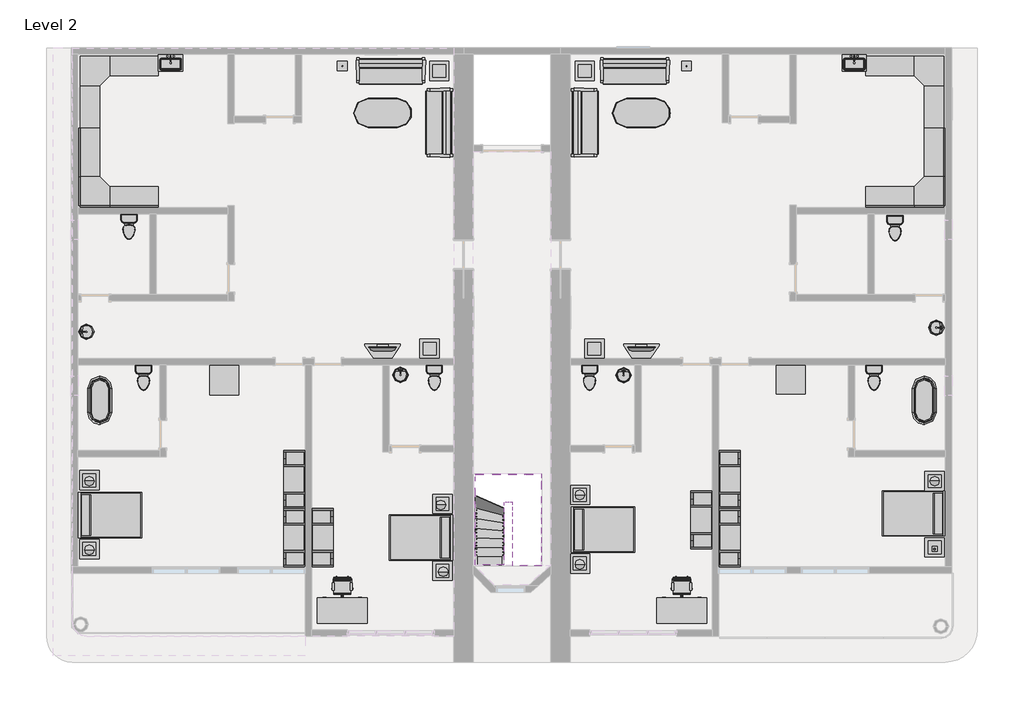
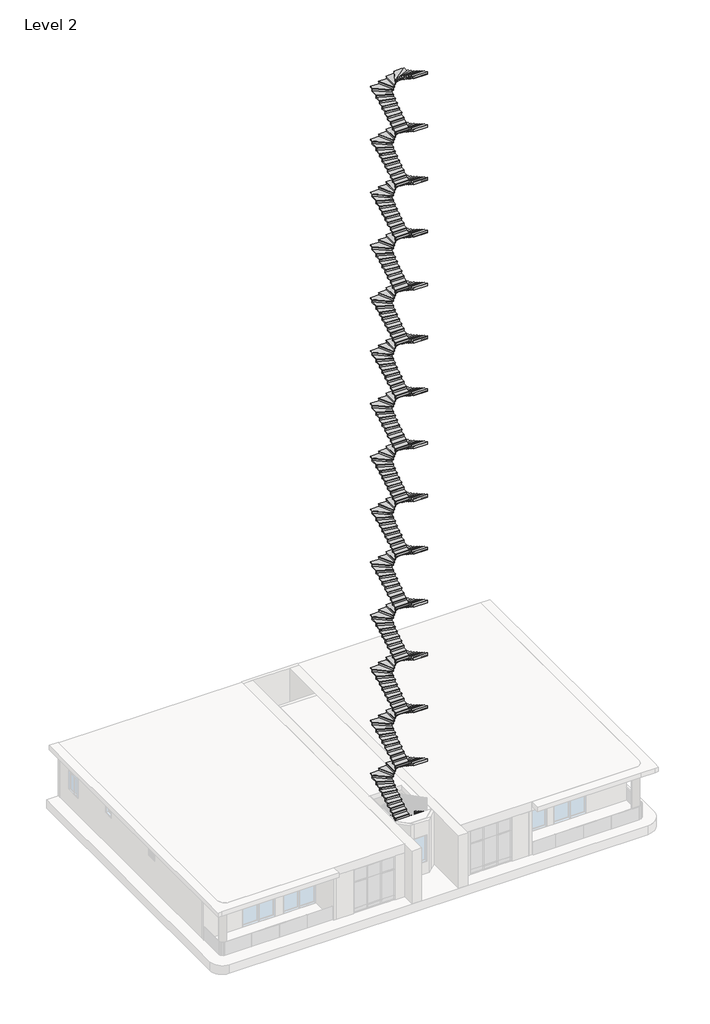
# One storey, part 5 of 5: 42 furniture elements, 16 stair flights, 14 flow terminals, 10 light fixtures.
"""IFC4 building model written with IfcOpenShell, lengths in millimetres."""

from ifc_helpers import new_model, si_unit, origin, place, context, project, spatial, transform, mapped, element, save
from components import flow_terminal_38af2918, flow_terminal_d49f872f, toilet_domestic_3d_toilet_domestic_3d_f7549cf7, toilet_domestic_3d_toilet_domestic_3d_183bbd19, flow_terminal_b374fae2, furniture_07436f11, furniture_096e7f55, chair_task_arms_chair_task_arms_fa5a08ef, furniture_072f6425, furniture_cf0b6580, furniture_aff9b2fb, furniture_56245f3a, tv_stand_tv_stand_6ce107e5, furniture_b5c51a22, furniture_2c34a4f9, furniture_4d44e21c, furniture_45e3acac, light_fixture_100w_120v_8564026f, table_lamp_hemispheric_60w_120v_02721d88, stair_flight_836873dd, stair_flight_696a7c4e, stair_flight_777e5497, stair_flight_57db1963, stair_flight_2efad17c, stair_flight_652fc51c, stair_flight_77a7b7b7, stair_flight_6c5b5e9d, stair_flight_464fb83d, stair_flight_aac49ba0, stair_flight_d4b8cc4c, stair_flight_2169dd6b, stair_flight_c7d98fdd, stair_flight_11ab74ad, stair_flight_b3d82c80

model = new_model("IFC4")

# Units and contexts
model_context = context("Model", 3, world=origin())
ifc_project = project(units=[si_unit("LENGTHUNIT", "METRE", prefix="MILLI")], contexts=[model_context])

# Site, building, storey
site = spatial("IfcSite", under=ifc_project)
building = spatial("IfcBuilding", under=site)
storey = spatial("IfcBuildingStorey", under=building, Name="Level 2", Elevation=3657.6)

# Flow terminals
placement = place(None, origin())
flow_terminal_shape = flow_terminal_38af2918(model_context)
element("IfcFlowTerminal", 1, ObjectType="Sink Kitchen-Single : 30\" x 21\"", at=placement, inside=storey, context=model_context, shape_type="MappedRepresentation", body=[
    mapped(flow_terminal_shape, transform((-15540.388011, 11239.7304546, 3657.6), x_axis=(1.0, 0.0, 0.0), y_axis=(0.0, 1.0, 0.0), z_axis=(0.0, 0.0, 1.0))),
])
element("IfcFlowTerminal", 2, ObjectType="Sink Kitchen-Single : 30\" x 21\"", at=placement, inside=storey, context=model_context, shape_type="MappedRepresentation", body=[
    mapped(flow_terminal_shape, transform((5948.011989, 11239.7304546, 3657.6), x_axis=(1.0, 0.0, 0.0), y_axis=(0.0, 1.0, 0.0), z_axis=(0.0, 0.0, 1.0))),
])
flow_terminal_2_shape = flow_terminal_d49f872f(model_context)
element("IfcFlowTerminal", 3, ObjectType="Sink Vanity-Round : 19\" x 19\"", at=placement, inside=storey, context=model_context, shape_type="MappedRepresentation", body=[
    mapped(flow_terminal_2_shape, transform((-18084.6070794, 2687.2241152, 3657.6), x_axis=(0.0, 1.0000000000000002, 0.0), y_axis=(-1.0000000000000002, 0.0, 0.0), z_axis=(0.0, 0.0, 1.0))),
])
element("IfcFlowTerminal", 4, ObjectType="Sink Vanity-Round : 19\" x 19\"", at=placement, inside=storey, context=model_context, shape_type="MappedRepresentation", body=[
    mapped(flow_terminal_2_shape, transform((8462.2249463, 3007.5275963, 3657.6), x_axis=(0.0, -1.0000000000000004, 0.0), y_axis=(1.0000000000000004, 0.0, 0.0), z_axis=(0.0, 0.0, 1.0))),
])
element("IfcFlowTerminal", 5, ObjectType="Sink Vanity-Round : 19\" x 19\"", at=placement, inside=storey, context=model_context, shape_type="MappedRepresentation", body=[
    mapped(flow_terminal_2_shape, transform((-8395.050511, 1341.8921141, 3657.6), x_axis=(1.0, 0.0, 0.0), y_axis=(0.0, 1.0, 0.0), z_axis=(0.0, 0.0, 1.0))),
])
element("IfcFlowTerminal", 6, ObjectType="Sink Vanity-Round : 19\" x 19\"", at=placement, inside=storey, context=model_context, shape_type="MappedRepresentation", body=[
    mapped(flow_terminal_2_shape, transform((-1384.650511, 1331.0855344, 3657.6), x_axis=(1.0, 0.0, 0.0), y_axis=(0.0, 1.0, 0.0), z_axis=(0.0, 0.0, 1.0))),
])
toilet_domestic_3d_toilet_domestic_3d_shape = toilet_domestic_3d_toilet_domestic_3d_f7549cf7(model_context)
toilet_domestic_3d_toilet_domestic_3d_2_shape = toilet_domestic_3d_toilet_domestic_3d_183bbd19(model_context)
element("IfcFlowTerminal", 7, ObjectType="Toilet-Domestic-3D : Toilet-Domestic-3D", at=placement, inside=storey, context=model_context, shape_type="MappedRepresentation", body=[
    mapped(toilet_domestic_3d_toilet_domestic_3d_shape, transform((6586.0012296, 1247.7798284, 3657.6), x_axis=(1.0, 0.0, 0.0), y_axis=(0.0, 1.0, 0.0), z_axis=(0.0, 0.0, 1.0))),
    mapped(toilet_domestic_3d_toilet_domestic_3d_2_shape, transform((6586.0012296, 1247.7798284, 3657.6), x_axis=(1.0, 0.0, 0.0), y_axis=(0.0, 1.0, 0.0), z_axis=(0.0, 0.0, 1.0))),
])
element("IfcFlowTerminal", 8, ObjectType="Toilet-Domestic-3D : Toilet-Domestic-3D", at=placement, inside=storey, context=model_context, shape_type="MappedRepresentation", body=[
    mapped(toilet_domestic_3d_toilet_domestic_3d_shape, transform((-2354.7987704, 1247.7798284, 3657.6), x_axis=(1.0, 0.0, 0.0), y_axis=(0.0, 1.0, 0.0), z_axis=(0.0, 0.0, 1.0))),
    mapped(toilet_domestic_3d_toilet_domestic_3d_2_shape, transform((-2354.7987704, 1247.7798284, 3657.6), x_axis=(1.0, 0.0, 0.0), y_axis=(0.0, 1.0, 0.0), z_axis=(0.0, 0.0, 1.0))),
])
element("IfcFlowTerminal", 9, ObjectType="Toilet-Domestic-3D : Toilet-Domestic-3D", at=placement, inside=storey, context=model_context, shape_type="MappedRepresentation", body=[
    mapped(toilet_domestic_3d_toilet_domestic_3d_shape, transform((-16375.5987704, 1247.7798284, 3657.6), x_axis=(1.0, 0.0, 0.0), y_axis=(0.0, 1.0, 0.0), z_axis=(0.0, 0.0, 1.0))),
    mapped(toilet_domestic_3d_toilet_domestic_3d_2_shape, transform((-16375.5987704, 1247.7798284, 3657.6), x_axis=(1.0, 0.0, 0.0), y_axis=(0.0, 1.0, 0.0), z_axis=(0.0, 0.0, 1.0))),
])
element("IfcFlowTerminal", 10, ObjectType="Toilet-Domestic-3D : Toilet-Domestic-3D", at=placement, inside=storey, context=model_context, shape_type="MappedRepresentation", body=[
    mapped(toilet_domestic_3d_toilet_domestic_3d_shape, transform((-16832.7987704, 5997.5798284, 3657.6), x_axis=(1.0, 0.0, 0.0), y_axis=(0.0, 1.0, 0.0), z_axis=(0.0, 0.0, 1.0))),
    mapped(toilet_domestic_3d_toilet_domestic_3d_2_shape, transform((-16832.7987704, 5997.5798284, 3657.6), x_axis=(1.0, 0.0, 0.0), y_axis=(0.0, 1.0, 0.0), z_axis=(0.0, 0.0, 1.0))),
])
element("IfcFlowTerminal", 11, ObjectType="Toilet-Domestic-3D : Toilet-Domestic-3D", at=placement, inside=storey, context=model_context, shape_type="MappedRepresentation", body=[
    mapped(toilet_domestic_3d_toilet_domestic_3d_shape, transform((7246.4012296, 5946.7798284, 3657.6), x_axis=(1.0, 0.0, 0.0), y_axis=(0.0, 1.0, 0.0), z_axis=(0.0, 0.0, 1.0))),
    mapped(toilet_domestic_3d_toilet_domestic_3d_2_shape, transform((7246.4012296, 5946.7798284, 3657.6), x_axis=(1.0, 0.0, 0.0), y_axis=(0.0, 1.0, 0.0), z_axis=(0.0, 0.0, 1.0))),
])
element("IfcFlowTerminal", 12, ObjectType="Toilet-Domestic-3D : Toilet-Domestic-3D", at=placement, inside=storey, context=model_context, shape_type="MappedRepresentation", body=[
    mapped(toilet_domestic_3d_toilet_domestic_3d_shape, transform((-7231.5987704, 1247.7798284, 3657.6), x_axis=(1.0, 0.0, 0.0), y_axis=(0.0, 1.0, 0.0), z_axis=(0.0, 0.0, 1.0))),
    mapped(toilet_domestic_3d_toilet_domestic_3d_2_shape, transform((-7231.5987704, 1247.7798284, 3657.6), x_axis=(1.0, 0.0, 0.0), y_axis=(0.0, 1.0, 0.0), z_axis=(0.0, 0.0, 1.0))),
])
flow_terminal_3_shape = flow_terminal_b374fae2(model_context)
element("IfcFlowTerminal", 13, ObjectType="Tub-Free Standing-3D : 30\" x 60\"", at=placement, inside=storey, context=model_context, shape_type="MappedRepresentation", body=[
    mapped(flow_terminal_3_shape, transform((-17747.1987704, 624.8758558, 3657.6), x_axis=(1.0, 0.0, 0.0), y_axis=(0.0, 1.0, 0.0), z_axis=(0.0, 0.0, 1.0))),
])
element("IfcFlowTerminal", 14, ObjectType="Tub-Free Standing-3D : 30\" x 60\"", at=placement, inside=storey, context=model_context, shape_type="MappedRepresentation", body=[
    mapped(flow_terminal_3_shape, transform((8160.8012296, 624.8758558, 3657.6), x_axis=(1.0, 0.0, 0.0), y_axis=(0.0, 1.0, 0.0), z_axis=(0.0, 0.0, 1.0))),
])

# Furniture
furniture_shape = furniture_07436f11(model_context)
element("IfcFurniture", 15, ObjectType="96\" x 96\"", at=placement, inside=storey, context=model_context, shape_type="MappedRepresentation", body=[
    mapped(furniture_shape, transform((-18275.8670182, 11991.0988634, 3657.6), x_axis=(1.0, 0.0, 0.0), y_axis=(0.0, 1.0, 0.0), z_axis=(0.0, 0.0, 1.0))),
])
element("IfcFurniture", 16, ObjectType="96\" x 96\"", at=placement, inside=storey, context=model_context, shape_type="MappedRepresentation", body=[
    mapped(furniture_shape, transform((9316.2242372, 11364.3441035, 3657.6), x_axis=(0.0, -1.0000000000000004, 0.0), y_axis=(1.0000000000000004, 0.0, 0.0), z_axis=(0.0, 0.0, 1.0))),
])
furniture_2_shape = furniture_096e7f55(model_context)
element("IfcFurniture", 17, ObjectType="Bed-Shaker : Double 56\" x 78\"", at=placement, inside=storey, context=model_context, shape_type="MappedRepresentation", body=[
    mapped(furniture_2_shape, transform((-18407.5987704, -2962.8741442, 3657.6), x_axis=(0.0, 1.0, 0.0), y_axis=(-1.0, 0.0, 0.0), z_axis=(0.0, 0.0, 1.0))),
])
element("IfcFurniture", 18, ObjectType="Bed-Shaker : Double 56\" x 78\"", at=placement, inside=storey, context=model_context, shape_type="MappedRepresentation", body=[
    mapped(furniture_2_shape, transform((-6672.7987704, -3712.1741442, 3657.6), x_axis=(0.0, -1.0, 0.0), y_axis=(1.0, 0.0, 0.0), z_axis=(0.0, 0.0, 1.0))),
])
element("IfcFurniture", 19, ObjectType="Bed-Shaker : Double 56\" x 78\"", at=placement, inside=storey, context=model_context, shape_type="MappedRepresentation", body=[
    mapped(furniture_2_shape, transform((-2913.5987704, -3420.0741442, 3657.6), x_axis=(0.0, 1.0000000000000002, 0.0), y_axis=(-1.0000000000000002, 0.0, 0.0), z_axis=(0.0, 0.0, 1.0))),
])
element("IfcFurniture", 20, ObjectType="Bed-Shaker : Double 56\" x 78\"", at=placement, inside=storey, context=model_context, shape_type="MappedRepresentation", body=[
    mapped(furniture_2_shape, transform((8821.2012296, -2950.1741442, 3657.6), x_axis=(0.0, -1.0, 0.0), y_axis=(1.0, 0.0, 0.0), z_axis=(0.0, 0.0, 1.0))),
])
chair_task_arms_chair_task_arms_shape = chair_task_arms_chair_task_arms_fa5a08ef(model_context)
element("IfcFurniture", 21, ObjectType="Chair-Task Arms : Chair-Task Arms", at=placement, inside=storey, context=model_context, shape_type="MappedRepresentation", body=[
    mapped(chair_task_arms_chair_task_arms_shape, transform((681.7920493, -5184.3566833, 3657.6), x_axis=(-1.0000000000000002, 0.0, 0.0), y_axis=(0.0, -1.0000000000000002, 0.0), z_axis=(0.0, 0.0, 1.0))),
])
element("IfcFurniture", 22, ObjectType="Chair-Task Arms : Chair-Task Arms", at=placement, inside=storey, context=model_context, shape_type="MappedRepresentation", body=[
    mapped(chair_task_arms_chair_task_arms_shape, transform((-9986.2079507, -5184.3566833, 3657.6), x_axis=(-1.0, 0.0, 0.0), y_axis=(0.0, -1.0, 0.0), z_axis=(0.0, 0.0, 1.0))),
])
furniture_3_shape = furniture_072f6425(model_context)
element("IfcFurniture", 23, ObjectType="Desk : 60\" x 30\"", at=placement, inside=storey, context=model_context, shape_type="MappedRepresentation", body=[
    mapped(furniture_3_shape, transform((-10889.1987704, -6371.702585, 3657.6), x_axis=(1.0, 0.0, 0.0), y_axis=(0.0, 1.0, 0.0), z_axis=(0.0, 0.0, 1.0))),
])
element("IfcFurniture", 24, ObjectType="Desk : 60\" x 30\"", at=placement, inside=storey, context=model_context, shape_type="MappedRepresentation", body=[
    mapped(furniture_3_shape, transform((-221.1987704, -6371.702585, 3657.6), x_axis=(1.0, 0.0, 0.0), y_axis=(0.0, 1.0, 0.0), z_axis=(0.0, 0.0, 1.0))),
])
furniture_4_shape = furniture_cf0b6580(model_context)
element("IfcFurniture", 25, ObjectType="Entertainment Center : 72\" x 72\" x 24\"", at=placement, inside=storey, context=model_context, shape_type="MappedRepresentation", body=[
    mapped(furniture_4_shape, transform((1607.6012296, -3134.3241442, 3657.6), x_axis=(0.0, -1.0000000000000002, 0.0), y_axis=(1.0000000000000002, 0.0, 0.0), z_axis=(0.0, 0.0, 1.0))),
])
element("IfcFurniture", 26, ObjectType="Entertainment Center : 72\" x 72\" x 24\"", at=placement, inside=storey, context=model_context, shape_type="MappedRepresentation", body=[
    mapped(furniture_4_shape, transform((1607.6012296, -3693.1241442, 3657.6), x_axis=(0.0, 1.0000000000000004, 0.0), y_axis=(-1.0000000000000004, 0.0, 0.0), z_axis=(0.0, 0.0, 1.0))),
])
element("IfcFurniture", 27, ObjectType="Entertainment Center : 72\" x 72\" x 24\"", at=placement, inside=storey, context=model_context, shape_type="MappedRepresentation", body=[
    mapped(furniture_4_shape, transform((1607.6012296, -1864.3241442, 3657.6), x_axis=(0.0, 1.0000000000000004, 0.0), y_axis=(-1.0000000000000004, 0.0, 0.0), z_axis=(0.0, 0.0, 1.0))),
])
element("IfcFurniture", 28, ObjectType="Entertainment Center : 72\" x 72\" x 24\"", at=placement, inside=storey, context=model_context, shape_type="MappedRepresentation", body=[
    mapped(furniture_4_shape, transform((-11193.9987704, -3693.1241442, 3657.6), x_axis=(0.0, -1.0000000000000016, 0.0), y_axis=(1.0000000000000016, 0.0, 0.0), z_axis=(0.0, 0.0, 1.0))),
])
element("IfcFurniture", 29, ObjectType="Entertainment Center : 72\" x 72\" x 24\"", at=placement, inside=storey, context=model_context, shape_type="MappedRepresentation", body=[
    mapped(furniture_4_shape, transform((-11193.9987704, -1864.3241442, 3657.6), x_axis=(0.0, -1.0000000000000004, 0.0), y_axis=(1.0000000000000004, 0.0, 0.0), z_axis=(0.0, 0.0, 1.0))),
])
element("IfcFurniture", 30, ObjectType="Entertainment Center : 72\" x 72\" x 24\"", at=placement, inside=storey, context=model_context, shape_type="MappedRepresentation", body=[
    mapped(furniture_4_shape, transform((-11193.9987704, -3693.1241442, 3657.6), x_axis=(0.0, 1.0, 0.0), y_axis=(-1.0, 0.0, 0.0), z_axis=(0.0, 0.0, 1.0))),
])
furniture_5_shape = furniture_aff9b2fb(model_context)
element("IfcFurniture", 31, ObjectType="Sofa-Pensi : 84\"", at=placement, inside=storey, context=model_context, shape_type="MappedRepresentation", body=[
    mapped(furniture_5_shape, transform((-8881.8050204, 10710.9660197, 3657.6), x_axis=(1.0, 0.0, 0.0), y_axis=(0.0, 1.0, 0.0), z_axis=(0.0, 0.0, 1.0))),
])
element("IfcFurniture", 32, ObjectType="Sofa-Pensi : 84\"", at=placement, inside=storey, context=model_context, shape_type="MappedRepresentation", body=[
    mapped(furniture_5_shape, transform((-7356.3086065, 9641.0821058, 3657.6), x_axis=(0.0, -1.0000000000000004, 0.0), y_axis=(1.0000000000000004, 0.0, 0.0), z_axis=(0.0, 0.0, 1.0))),
])
element("IfcFurniture", 33, ObjectType="Sofa-Pensi : 84\"", at=placement, inside=storey, context=model_context, shape_type="MappedRepresentation", body=[
    mapped(furniture_5_shape, transform((-2230.0889343, 9083.8696058, 3657.6), x_axis=(0.0, 1.0000000000000002, 0.0), y_axis=(-1.0000000000000002, 0.0, 0.0), z_axis=(0.0, 0.0, 1.0))),
])
element("IfcFurniture", 34, ObjectType="Sofa-Pensi : 84\"", at=placement, inside=storey, context=model_context, shape_type="MappedRepresentation", body=[
    mapped(furniture_5_shape, transform((-1211.0050204, 10710.9660197, 3657.6), x_axis=(1.0000000000000007, 0.0, 0.0), y_axis=(0.0, 1.0000000000000007, 0.0), z_axis=(0.0, 0.0, 1.0))),
])
furniture_6_shape = furniture_56245f3a(model_context)
element("IfcFurniture", 35, ObjectType="TV - Flat Screen : 32\"", at=placement, inside=storey, context=model_context, shape_type="MappedRepresentation", body=[
    mapped(furniture_6_shape, transform((-8861.1432846, 2232.8144794, 4572.0), x_axis=(-1.0, 0.0, 0.0), y_axis=(0.0, -1.0, 0.0), z_axis=(0.0, 0.0, 1.0))),
])
element("IfcFurniture", 36, ObjectType="TV - Flat Screen : 32\"", at=placement, inside=storey, context=model_context, shape_type="MappedRepresentation", body=[
    mapped(furniture_6_shape, transform((-733.1432846, 2232.8144794, 4572.0), x_axis=(-1.0, 0.0, 0.0), y_axis=(0.0, -1.0, 0.0), z_axis=(0.0, 0.0, 1.0))),
])
tv_stand_tv_stand_shape = tv_stand_tv_stand_6ce107e5(model_context)
element("IfcFurniture", 37, ObjectType="TV Stand : TV Stand", at=placement, inside=storey, context=model_context, shape_type="MappedRepresentation", body=[
    mapped(tv_stand_tv_stand_shape, transform((-8732.0107683, 1945.6758558, 3657.6), x_axis=(-1.0000000000000002, 0.0, 0.0), y_axis=(0.0, -1.0000000000000002, 0.0), z_axis=(0.0, 0.0, 1.0))),
])
element("IfcFurniture", 38, ObjectType="TV Stand : TV Stand", at=placement, inside=storey, context=model_context, shape_type="MappedRepresentation", body=[
    mapped(tv_stand_tv_stand_shape, transform((-604.0107683, 1945.6758558, 3657.6), x_axis=(-1.0, 0.0, 0.0), y_axis=(0.0, -1.0, 0.0), z_axis=(0.0, 0.0, 1.0))),
])
furniture_7_shape = furniture_b5c51a22(model_context)
element("IfcFurniture", 39, ObjectType="Table-Coffee : 24\" x 24\" x 24\"", at=placement, inside=storey, context=model_context, shape_type="MappedRepresentation", body=[
    mapped(furniture_7_shape, transform((-7097.4645371, 10892.864778, 3657.6), x_axis=(1.0, 0.0, 0.0), y_axis=(0.0, 1.0, 0.0), z_axis=(0.0, 0.0, 1.0))),
])
element("IfcFurniture", 40, ObjectType="Table-Coffee : 24\" x 24\" x 24\"", at=placement, inside=storey, context=model_context, shape_type="MappedRepresentation", body=[
    mapped(furniture_7_shape, transform((-2525.4645371, 10892.864778, 3657.6), x_axis=(1.0, 0.0, 0.0), y_axis=(0.0, 1.0, 0.0), z_axis=(0.0, 0.0, 1.0))),
])
element("IfcFurniture", 41, ObjectType="Table-Coffee : 24\" x 24\" x 24\"", at=placement, inside=storey, context=model_context, shape_type="MappedRepresentation", body=[
    mapped(furniture_7_shape, transform((-7402.2645371, 2155.264778, 3657.6), x_axis=(1.0, 0.0, 0.0), y_axis=(0.0, 1.0, 0.0), z_axis=(0.0, 0.0, 1.0))),
])
element("IfcFurniture", 42, ObjectType="Table-Coffee : 24\" x 24\" x 24\"", at=placement, inside=storey, context=model_context, shape_type="MappedRepresentation", body=[
    mapped(furniture_7_shape, transform((-2220.6645371, 2155.264778, 3657.6), x_axis=(1.0, 0.0, 0.0), y_axis=(0.0, 1.0, 0.0), z_axis=(0.0, 0.0, 1.0))),
])
element("IfcFurniture", 43, ObjectType="Table-Coffee : 24\" x 24\" x 24\"", at=placement, inside=storey, context=model_context, shape_type="MappedRepresentation", body=[
    mapped(furniture_7_shape, transform((-2677.8645371, -4601.135222, 3657.6), x_axis=(1.0, 0.0, 0.0), y_axis=(0.0, 1.0, 0.0), z_axis=(0.0, 0.0, 1.0))),
])
element("IfcFurniture", 44, ObjectType="Table-Coffee : 24\" x 24\" x 24\"", at=placement, inside=storey, context=model_context, shape_type="MappedRepresentation", body=[
    mapped(furniture_7_shape, transform((-18095.6645371, -4143.935222, 3657.6), x_axis=(1.0, 0.0, 0.0), y_axis=(0.0, 1.0, 0.0), z_axis=(0.0, 0.0, 1.0))),
])
element("IfcFurniture", 45, ObjectType="Table-Coffee : 24\" x 24\" x 24\"", at=placement, inside=storey, context=model_context, shape_type="MappedRepresentation", body=[
    mapped(furniture_7_shape, transform((-18095.6645371, -1984.935222, 3657.6), x_axis=(1.0, 0.0, 0.0), y_axis=(0.0, 1.0, 0.0), z_axis=(0.0, 0.0, 1.0))),
])
element("IfcFurniture", 46, ObjectType="Table-Coffee : 24\" x 24\" x 24\"", at=placement, inside=storey, context=model_context, shape_type="MappedRepresentation", body=[
    mapped(furniture_7_shape, transform((-2677.8645371, -2442.135222, 3657.6), x_axis=(1.0, 0.0, 0.0), y_axis=(0.0, 1.0, 0.0), z_axis=(0.0, 0.0, 1.0))),
])
element("IfcFurniture", 47, ObjectType="Table-Coffee : 24\" x 24\" x 24\"", at=placement, inside=storey, context=model_context, shape_type="MappedRepresentation", body=[
    mapped(furniture_7_shape, transform((8472.7354629, -4093.135222, 3657.6), x_axis=(1.0, 0.0, 0.0), y_axis=(0.0, 1.0, 0.0), z_axis=(0.0, 0.0, 1.0))),
])
element("IfcFurniture", 48, ObjectType="Table-Coffee : 24\" x 24\" x 24\"", at=placement, inside=storey, context=model_context, shape_type="MappedRepresentation", body=[
    mapped(furniture_7_shape, transform((8472.7354629, -2010.335222, 3657.6), x_axis=(1.0, 0.0, 0.0), y_axis=(0.0, 1.0, 0.0), z_axis=(0.0, 0.0, 1.0))),
])
element("IfcFurniture", 49, ObjectType="Table-Coffee : 24\" x 24\" x 24\"", at=placement, inside=storey, context=model_context, shape_type="MappedRepresentation", body=[
    mapped(furniture_7_shape, transform((-6995.8645371, -4832.0414601, 3657.6), x_axis=(1.0, 0.0, 0.0), y_axis=(0.0, 1.0, 0.0), z_axis=(0.0, 0.0, 1.0))),
])
element("IfcFurniture", 50, ObjectType="Table-Coffee : 24\" x 24\" x 24\"", at=placement, inside=storey, context=model_context, shape_type="MappedRepresentation", body=[
    mapped(furniture_7_shape, transform((-6995.8645371, -2723.8414601, 3657.6), x_axis=(1.0, 0.0, 0.0), y_axis=(0.0, 1.0, 0.0), z_axis=(0.0, 0.0, 1.0))),
])
furniture_8_shape = furniture_2c34a4f9(model_context)
element("IfcFurniture", 51, ObjectType="Table-Dining Oval : 36\" x 72\"", at=placement, inside=storey, context=model_context, shape_type="MappedRepresentation", body=[
    mapped(furniture_8_shape, transform((-8455.3790983, 10025.3742164, 3657.6), x_axis=(1.0, 0.0, 0.0), y_axis=(0.0, 1.0, 0.0), z_axis=(0.0, 0.0, 1.0))),
])
element("IfcFurniture", 52, ObjectType="Table-Dining Oval : 36\" x 72\"", at=placement, inside=storey, context=model_context, shape_type="MappedRepresentation", body=[
    mapped(furniture_8_shape, transform((-327.3790983, 10025.3742164, 3657.6), x_axis=(1.0, 0.0, 0.0), y_axis=(0.0, 1.0, 0.0), z_axis=(0.0, 0.0, 1.0))),
])
furniture_9_shape = furniture_4d44e21c(model_context)
element("IfcFurniture", 53, ObjectType="Table-Rectangular : 36\" x 36\"", at=placement, inside=storey, context=model_context, shape_type="MappedRepresentation", body=[
    mapped(furniture_9_shape, transform((-13835.5987704, 1259.8758558, 3657.6), x_axis=(1.0, 0.0, 0.0), y_axis=(0.0, 1.0, 0.0), z_axis=(0.0, 0.0, 1.0))),
])
element("IfcFurniture", 54, ObjectType="Table-Rectangular : 36\" x 36\"", at=placement, inside=storey, context=model_context, shape_type="MappedRepresentation", body=[
    mapped(furniture_9_shape, transform((3969.8012296, 1285.2758558, 3657.6), x_axis=(1.0, 0.0, 0.0), y_axis=(0.0, 1.0, 0.0), z_axis=(0.0, 0.0, 1.0))),
])
furniture_10_shape = furniture_45e3acac(model_context)
element("IfcFurniture", 55, ObjectType="Work Station Cubicle : 96\" x 96\"", at=placement, inside=storey, context=model_context, shape_type="MappedRepresentation", body=[
    mapped(furniture_10_shape, transform((-18902.621778, 6827.207608, 3657.6), x_axis=(0.0, 0.9999999999999999, 0.0), y_axis=(-0.9999999999999999, 0.0, 0.0), z_axis=(0.0, 0.0, 1.0))),
])
element("IfcFurniture", 56, ObjectType="Work Station Cubicle : 96\" x 96\"", at=placement, inside=storey, context=model_context, shape_type="MappedRepresentation", body=[
    mapped(furniture_10_shape, transform((8689.4694774, 6200.4528481, 3657.6), x_axis=(-1.0000000000000007, 0.0, 0.0), y_axis=(0.0, -1.0000000000000007, 0.0), z_axis=(0.0, 0.0, 1.0))),
])

# Light fixtures
light_fixture_100w_120v_shape = light_fixture_100w_120v_8564026f(model_context)
element("IfcLightFixture", 57, ObjectType="100W - 120V", at=placement, inside=storey, context=model_context, shape_type="MappedRepresentation", body=[
    mapped(light_fixture_100w_120v_shape, transform((-10127.1987704, 11140.4758558, 3657.6), x_axis=(1.0, 0.0, 0.0), y_axis=(0.0, 1.0, 0.0), z_axis=(0.0, 0.0, 1.0))),
])
element("IfcLightFixture", 58, ObjectType="100W - 120V", at=placement, inside=storey, context=model_context, shape_type="MappedRepresentation", body=[
    mapped(light_fixture_100w_120v_shape, transform((693.2012296, 11140.4758558, 3657.6), x_axis=(1.0, 0.0, 0.0), y_axis=(0.0, 1.0, 0.0), z_axis=(0.0, 0.0, 1.0))),
])
table_lamp_hemispheric_60w_120v_shape = table_lamp_hemispheric_60w_120v_02721d88(model_context)
element("IfcLightFixture", 59, ObjectType="Table Lamp - Hemispheric : 60W - 120V", at=placement, inside=storey, context=model_context, shape_type="MappedRepresentation", body=[
    mapped(table_lamp_hemispheric_60w_120v_shape, transform((-18077.3987704, -1915.1241442, 4267.2), x_axis=(1.0, 0.0, 0.0), y_axis=(0.0, 1.0, 0.0), z_axis=(0.0, 0.0, 1.0))),
])
element("IfcLightFixture", 60, ObjectType="Table Lamp - Hemispheric : 60W - 120V", at=placement, inside=storey, context=model_context, shape_type="MappedRepresentation", body=[
    mapped(table_lamp_hemispheric_60w_120v_shape, transform((-7028.3987704, -2666.7303823, 4267.2), x_axis=(1.0, 0.0, 0.0), y_axis=(0.0, 1.0, 0.0), z_axis=(0.0, 0.0, 1.0))),
])
element("IfcLightFixture", 61, ObjectType="Table Lamp - Hemispheric : 60W - 120V", at=placement, inside=storey, context=model_context, shape_type="MappedRepresentation", body=[
    mapped(table_lamp_hemispheric_60w_120v_shape, transform((-2659.5987704, -2346.9241442, 4267.2), x_axis=(1.0, 0.0, 0.0), y_axis=(0.0, 1.0, 0.0), z_axis=(0.0, 0.0, 1.0))),
])
element("IfcLightFixture", 62, ObjectType="Table Lamp - Hemispheric : 60W - 120V", at=placement, inside=storey, context=model_context, shape_type="MappedRepresentation", body=[
    mapped(table_lamp_hemispheric_60w_120v_shape, transform((8491.0012296, -4048.7241442, 4572.0), x_axis=(1.0, 0.0, 0.0), y_axis=(0.0, 1.0, 0.0), z_axis=(0.0, 0.0, 1.0))),
])
element("IfcLightFixture", 63, ObjectType="Table Lamp - Hemispheric : 60W - 120V", at=placement, inside=storey, context=model_context, shape_type="MappedRepresentation", body=[
    mapped(table_lamp_hemispheric_60w_120v_shape, transform((8491.0012296, -1915.1241442, 4267.2), x_axis=(1.0, 0.0, 0.0), y_axis=(0.0, 1.0, 0.0), z_axis=(0.0, 0.0, 1.0))),
])
element("IfcLightFixture", 64, ObjectType="Table Lamp - Hemispheric : 60W - 120V", at=placement, inside=storey, context=model_context, shape_type="MappedRepresentation", body=[
    mapped(table_lamp_hemispheric_60w_120v_shape, transform((-2659.5987704, -4531.3241442, 4267.2), x_axis=(1.0, 0.0, 0.0), y_axis=(0.0, 1.0, 0.0), z_axis=(0.0, 0.0, 1.0))),
])
element("IfcLightFixture", 65, ObjectType="Table Lamp - Hemispheric : 60W - 120V", at=placement, inside=storey, context=model_context, shape_type="MappedRepresentation", body=[
    mapped(table_lamp_hemispheric_60w_120v_shape, transform((-6952.1987704, -4762.2303823, 4267.2), x_axis=(1.0, 0.0, 0.0), y_axis=(0.0, 1.0, 0.0), z_axis=(0.0, 0.0, 1.0))),
])
element("IfcLightFixture", 66, ObjectType="Table Lamp - Hemispheric : 60W - 120V", at=placement, inside=storey, context=model_context, shape_type="MappedRepresentation", body=[
    mapped(table_lamp_hemispheric_60w_120v_shape, transform((-18077.3987704, -4074.1241442, 4267.2), x_axis=(1.0, 0.0, 0.0), y_axis=(0.0, 1.0, 0.0), z_axis=(0.0, 0.0, 1.0))),
])

# Stair flights
stair_flight_shape = stair_flight_836873dd(model_context)
element("IfcStairFlight", 67, ObjectType="2\" Tread 1\" Nosing 1/4\" Riser", at=placement, inside=storey, context=model_context, shape_type="MappedRepresentation", body=[
    mapped(stair_flight_shape, transform((0.0, 0.0, 0.0), x_axis=(1.0, 0.0, 0.0), y_axis=(0.0, 1.0, 0.0), z_axis=(0.0, 0.0, 1.0))),
])
stair_flight_2_shape = stair_flight_696a7c4e(model_context)
element("IfcStairFlight", 68, ObjectType="2\" Tread 1\" Nosing 1/4\" Riser", at=placement, inside=storey, context=model_context, shape_type="MappedRepresentation", body=[
    mapped(stair_flight_2_shape, transform((0.0, 0.0, 0.0), x_axis=(1.0, 0.0, 0.0), y_axis=(0.0, 1.0, 0.0), z_axis=(0.0, 0.0, 1.0))),
])
stair_flight_3_shape = stair_flight_777e5497(model_context)
element("IfcStairFlight", 69, ObjectType="2\" Tread 1\" Nosing 1/4\" Riser", at=placement, inside=storey, context=model_context, shape_type="MappedRepresentation", body=[
    mapped(stair_flight_3_shape, transform((0.0, 0.0, 0.0), x_axis=(1.0, 0.0, 0.0), y_axis=(0.0, 1.0, 0.0), z_axis=(0.0, 0.0, 1.0))),
])
stair_flight_4_shape = stair_flight_57db1963(model_context)
element("IfcStairFlight", 70, ObjectType="2\" Tread 1\" Nosing 1/4\" Riser", at=placement, inside=storey, context=model_context, shape_type="MappedRepresentation", body=[
    mapped(stair_flight_4_shape, transform((0.0, 0.0, 0.0), x_axis=(1.0, 0.0, 0.0), y_axis=(0.0, 1.0, 0.0), z_axis=(0.0, 0.0, 1.0))),
])
stair_flight_5_shape = stair_flight_2efad17c(model_context)
element("IfcStairFlight", 71, ObjectType="2\" Tread 1\" Nosing 1/4\" Riser", at=placement, inside=storey, context=model_context, shape_type="MappedRepresentation", body=[
    mapped(stair_flight_5_shape, transform((0.0, 0.0, 0.0), x_axis=(1.0, 0.0, 0.0), y_axis=(0.0, 1.0, 0.0), z_axis=(0.0, 0.0, 1.0))),
])
stair_flight_6_shape = stair_flight_652fc51c(model_context)
element("IfcStairFlight", 72, ObjectType="2\" Tread 1\" Nosing 1/4\" Riser", at=placement, inside=storey, context=model_context, shape_type="MappedRepresentation", body=[
    mapped(stair_flight_6_shape, transform((0.0, 0.0, 0.0), x_axis=(1.0, 0.0, 0.0), y_axis=(0.0, 1.0, 0.0), z_axis=(0.0, 0.0, 1.0))),
])
element("IfcStairFlight", 73, ObjectType="2\" Tread 1\" Nosing 1/4\" Riser", at=placement, inside=storey, context=model_context, shape_type="MappedRepresentation", body=[
    mapped(stair_flight_6_shape, transform((0.0, 0.0, 0.0), x_axis=(1.0, 0.0, 0.0), y_axis=(0.0, 1.0, 0.0), z_axis=(0.0, 0.0, 1.0))),
])
stair_flight_7_shape = stair_flight_77a7b7b7(model_context)
element("IfcStairFlight", 74, ObjectType="2\" Tread 1\" Nosing 1/4\" Riser", at=placement, inside=storey, context=model_context, shape_type="MappedRepresentation", body=[
    mapped(stair_flight_7_shape, transform((0.0, 0.0, 0.0), x_axis=(1.0, 0.0, 0.0), y_axis=(0.0, 1.0, 0.0), z_axis=(0.0, 0.0, 1.0))),
])
stair_flight_8_shape = stair_flight_6c5b5e9d(model_context)
element("IfcStairFlight", 75, ObjectType="2\" Tread 1\" Nosing 1/4\" Riser", at=placement, inside=storey, context=model_context, shape_type="MappedRepresentation", body=[
    mapped(stair_flight_8_shape, transform((0.0, 0.0, 0.0), x_axis=(1.0, 0.0, 0.0), y_axis=(0.0, 1.0, 0.0), z_axis=(0.0, 0.0, 1.0))),
])
stair_flight_9_shape = stair_flight_464fb83d(model_context)
element("IfcStairFlight", 76, ObjectType="2\" Tread 1\" Nosing 1/4\" Riser", at=placement, inside=storey, context=model_context, shape_type="MappedRepresentation", body=[
    mapped(stair_flight_9_shape, transform((0.0, 0.0, 0.0), x_axis=(1.0, 0.0, 0.0), y_axis=(0.0, 1.0, 0.0), z_axis=(0.0, 0.0, 1.0))),
])
stair_flight_10_shape = stair_flight_aac49ba0(model_context)
element("IfcStairFlight", 77, ObjectType="2\" Tread 1\" Nosing 1/4\" Riser", at=placement, inside=storey, context=model_context, shape_type="MappedRepresentation", body=[
    mapped(stair_flight_10_shape, transform((0.0, 0.0, 0.0), x_axis=(1.0, 0.0, 0.0), y_axis=(0.0, 1.0, 0.0), z_axis=(0.0, 0.0, 1.0))),
])
stair_flight_11_shape = stair_flight_d4b8cc4c(model_context)
element("IfcStairFlight", 78, ObjectType="2\" Tread 1\" Nosing 1/4\" Riser", at=placement, inside=storey, context=model_context, shape_type="MappedRepresentation", body=[
    mapped(stair_flight_11_shape, transform((0.0, 0.0, 0.0), x_axis=(1.0, 0.0, 0.0), y_axis=(0.0, 1.0, 0.0), z_axis=(0.0, 0.0, 1.0))),
])
stair_flight_12_shape = stair_flight_2169dd6b(model_context)
element("IfcStairFlight", 79, ObjectType="2\" Tread 1\" Nosing 1/4\" Riser", at=placement, inside=storey, context=model_context, shape_type="MappedRepresentation", body=[
    mapped(stair_flight_12_shape, transform((0.0, 0.0, 0.0), x_axis=(1.0, 0.0, 0.0), y_axis=(0.0, 1.0, 0.0), z_axis=(0.0, 0.0, 1.0))),
])
stair_flight_13_shape = stair_flight_c7d98fdd(model_context)
element("IfcStairFlight", 80, ObjectType="2\" Tread 1\" Nosing 1/4\" Riser", at=placement, inside=storey, context=model_context, shape_type="MappedRepresentation", body=[
    mapped(stair_flight_13_shape, transform((0.0, 0.0, 0.0), x_axis=(1.0, 0.0, 0.0), y_axis=(0.0, 1.0, 0.0), z_axis=(0.0, 0.0, 1.0))),
])
stair_flight_14_shape = stair_flight_11ab74ad(model_context)
element("IfcStairFlight", 81, ObjectType="2\" Tread 1\" Nosing 1/4\" Riser", at=placement, inside=storey, context=model_context, shape_type="MappedRepresentation", body=[
    mapped(stair_flight_14_shape, transform((0.0, 0.0, 0.0), x_axis=(1.0, 0.0, 0.0), y_axis=(0.0, 1.0, 0.0), z_axis=(0.0, 0.0, 1.0))),
])
stair_flight_15_shape = stair_flight_b3d82c80(model_context)
element("IfcStairFlight", 82, ObjectType="2\" Tread 1\" Nosing 1/4\" Riser", at=placement, inside=storey, context=model_context, shape_type="MappedRepresentation", body=[
    mapped(stair_flight_15_shape, transform((0.0, 0.0, 0.0), x_axis=(1.0, 0.0, 0.0), y_axis=(0.0, 1.0, 0.0), z_axis=(0.0, 0.0, 1.0))),
])

save(model, "model.ifc")

# Revit data of these elements
# Type "Sink Kitchen-Single : 30\" x 21\""
#   Assembly Code = "D2010410"
#   Counter Height = 3' - 0"
#   Depth = 1' - 9"
#   Width = 2' - 6"
#   Faucet Material = Steel, Polished
#   Sink Material = Steel, Polished
# Type "Sink Vanity-Round : 19\" x 19\""
#   Assembly Code = "D2010400"
#   Top Of Counter = 2' - 7"
#   Basin Material = Porcelain, Linen
#   Faucet Material = Steel, Polished
# Type "Toilet-Domestic-3D : Toilet-Domestic-3D"
#   Assembly Code = "D2010110"
#   Toilet - Bowl/Basin Material = Porcelain, Linen
#   Toilet - Seat Material = Laminate, Linen, Matte
# Type "Tub-Free Standing-3D : 30\" x 60\""
#   Assembly Code = "D2010110"
#   Height = 1' - 6"
#   Length = 5' - 0"
#   Width = 2' - 6"
#   Tub Material = Porcelain, Ivory
# Type "96\" x 96\""
#   Assembly Code = "E2020"
#   Desktop Height = 2' - 6"
#   Desktop1 Width = 2' - 0"
#   Desktop2 Width = 2' - 0"
#   Panel1 Length = 5' - 0"
#   Panel2 Length = 5' - 0"
#   Work Top Material = Laminate, Ivory, Matte
# Type "Bed-Shaker : Double 56\" x 78\""
#   Assembly Code = "E2020200"
#   Length = 6' - 6"
#   Width = 4' - 8"
#   Frame Material = Birch
#   Mattress Material = Linen, White
# Type "Chair-Task Arms : Chair-Task Arms"
#   Assembly Code = "E2020200"
#   Base Material = Plastic, Opaque Black
#   Caster Material = Plastic, Opaque Black
#   Seat/Back Material = Textile - Slate Blue
# Type "Desk : 60\" x 30\""
#   Assembly Code = "E2020200"
#   Depth = 2' - 6"
#   Height = 2' - 6"
#   Leg Height = 0' - 6"
#   Width = 5' - 0"
#   Body Material = Laminate, Ivory, Matte
#   Handle/Leg Material = Steel, Chrome Plated
#   Top Material = Cherry
# Type "Entertainment Center : 72\" x 72\" x 24\""
#   Assembly Code = "E2020200"
#   Center Width = 2' - 8"
#   Depth = 2' - 0"
#   Height = 6' - 0"
#   Width = 6' - 0"
#   Material = none
# Type "Sofa-Pensi : 84\""
#   Assembly Code = "E2020200"
#   Length = 7' - 0"
#   Frame Material = Cherry
#   Seat Material = Linen, Beige
#   Feet Material = Steel, Chrome Plated
# Type "TV - Flat Screen : 32\""
#   SinAng = 0' - 0.0193"
#   L = 2' - 3.79372"
#   H = 1' - 3.6354"
#   Thickness = 0' - 4.33071"
#   Diagonal = 2' - 7.88976"
#   CosAng = 0' - 0.03431"
#   Stand [instance default] = yes
# Type "TV Stand : TV Stand"
#   Depth = 1' - 6"
#   Width = 3' - 8"
#   Height = 1' - 7 1/2"
#   Finish = Melamine - Gray
# Type "Table-Coffee : 24\" x 24\" x 24\""
#   Assembly Code = "E2020200"
#   Height = 2' - 0"
#   Length = 2' - 0"
#   Width = 2' - 0"
#   Top Material = none
#   Frame Material = none
# Type "Table-Dining Oval : 36\" x 72\""
#   Assembly Code = "E2020200"
#   Length = 6' - 0"
#   Width = 3' - 0"
#   Base Material = Steel, Chrome Plated
#   Top Material = Glass - Clear, Grey
#   Description = (empty or 0)
# Type "Table-Rectangular : 36\" x 36\""
#   Assembly Code = "E2020200"
#   Height = 2' - 6"
#   Length = 3' - 0"
#   Width = 3' - 0"
#   Base Material = Birch
#   Top Material = Birch
# Type "Work Station Cubicle : 96\" x 96\""
#   Assembly Code = "E2020"
#   Desktop Height = 2' - 6"
#   Desktop1 Width = 2' - 0"
#   Desktop2 Width = 2' - 0"
#   Panel Height = 5' - 6"
#   Panel1 Length = 5' - 0"
#   Panel2 Length = 5' - 0"
#   Cube Panel Material = Textile - Light Gray
#   Work Top Material = Laminate, Ivory, Matte
# Type "100W - 120V"
#   Assembly Code = "D5020220"
#   Lamp = "A-19"
#   Wattage Comments = "100"
#   Wattage = 100 W
#   built-in parameter 1150110 = 1 (stored number, unit not read)
#   built-in parameter 1114217 = 1 (stored number, unit not read)
#   built-in parameter 1150109 = 1 (stored number, unit not read)
#   built-in parameter 1150113 = 1 (stored number, unit not read)
#   built-in parameter 1150115 = 1 (stored number, unit not read)
#   built-in parameter 1150105 = 139.261 (stored number, unit not read)
#   Light Source Symbol Size = 2' - 0"
#   built-in parameter 1150112 = 1 (stored number, unit not read)
#   built-in parameter 1150114 = 1 (stored number, unit not read)
#   built-in parameter 1150107 = 2800 (stored number, unit not read)
#   built-in parameter 1150106 = 1.39261 (stored number, unit not read)
#   built-in parameter 1150104 = 1.6258 (stored number, unit not read)
#   Ballast Voltage = 120 V
#   built-in parameter 1114218 = 1 (stored number, unit not read)
#   built-in parameter 1150133 = 10 (stored number, unit not read)
#   Lumens = 1750 lm
#   Apparent Load = 100 VA
#   built-in parameter 1150134 = 4
#   built-in parameter 1150137 = 1
#   Color Filter = 16777215
#   Ballast Number of Poles = 1
#   Shade = Glass, Frosted
#   Stand = Steel, Chrome Plated
#   Dimming Lamp Color Temperature Shift = (empty or 0)
# Type "Table Lamp - Hemispheric : 60W - 120V"
#   Assembly Code = "D5020220"
#   Lamp = "A-19"
#   Wattage = 60 W
#   built-in parameter 1150110 = 1 (stored number, unit not read)
#   built-in parameter 1114217 = 1 (stored number, unit not read)
#   built-in parameter 1150109 = 1 (stored number, unit not read)
#   built-in parameter 1150113 = 1 (stored number, unit not read)
#   built-in parameter 1150115 = 1 (stored number, unit not read)
#   built-in parameter 1150105 = 68.0387 (stored number, unit not read)
#   Light Source Symbol Size = 2' - 0"
#   built-in parameter 1150112 = 1 (stored number, unit not read)
#   built-in parameter 1150114 = 1 (stored number, unit not read)
#   built-in parameter 1150107 = 2800 (stored number, unit not read)
#   built-in parameter 1150106 = 0.680387 (stored number, unit not read)
#   built-in parameter 1150104 = 1.32387 (stored number, unit not read)
#   Ballast Voltage = 120 V
#   built-in parameter 1114218 = 1 (stored number, unit not read)
#   built-in parameter 1150133 = 10 (stored number, unit not read)
#   Lumens = 855 lm
#   Apparent Load = 60 VA
#   built-in parameter 1150134 = 4
#   built-in parameter 1150137 = 1
#   Color Filter = 16777215
#   Ballast Number of Poles = 1
#   Mount Material = Steel, Chrome Plated
#   Shade Material = Glass, Frosted
#   Base Material = Birch
#   Dimming Lamp Color Temperature Shift = (empty or 0)
#   Wattage Comments = ""
# Element 1 (IfcFlowTerminal, "Sink Kitchen-Single : 30\" x 21\"")
#   Mark = "3"
#   Phase Created = New Construction
#   Materials on its faces: "Steel, Polished"
# Element 2 (IfcFlowTerminal, "Sink Kitchen-Single : 30\" x 21\"")
#   Mark = "4"
#   Phase Created = New Construction
#   Materials on its faces: "Steel, Polished"
# Element 3 (IfcFlowTerminal, "Sink Vanity-Round : 19\" x 19\"")
#   Mark = "7"
#   Phase Created = New Construction
#   Materials on its faces: "Porcelain, Linen", "Steel, Polished"
# Element 4 (IfcFlowTerminal, "Sink Vanity-Round : 19\" x 19\"")
#   Mark = "8"
#   Phase Created = New Construction
#   Materials on its faces: "Porcelain, Linen", "Steel, Polished"
# Element 5 (IfcFlowTerminal, "Sink Vanity-Round : 19\" x 19\"")
#   Mark = "19"
#   Phase Created = New Construction
#   Materials on its faces: "Porcelain, Linen", "Steel, Polished"
# Element 6 (IfcFlowTerminal, "Sink Vanity-Round : 19\" x 19\"")
#   Mark = "20"
#   Phase Created = New Construction
#   Materials on its faces: "Porcelain, Linen", "Steel, Polished"
# Element 7 (IfcFlowTerminal, "Toilet-Domestic-3D : Toilet-Domestic-3D")
#   Mark = "13"
#   Phase Created = New Construction
#   Materials on its faces: "Porcelain, Linen", "Laminate, Linen, Matte"
# Element 8 (IfcFlowTerminal, "Toilet-Domestic-3D : Toilet-Domestic-3D")
#   Mark = "14"
#   Phase Created = New Construction
#   Materials on its faces: "Porcelain, Linen", "Laminate, Linen, Matte"
# Element 9 (IfcFlowTerminal, "Toilet-Domestic-3D : Toilet-Domestic-3D")
#   Mark = "15"
#   Phase Created = New Construction
#   Materials on its faces: "Porcelain, Linen", "Laminate, Linen, Matte"
# Element 10 (IfcFlowTerminal, "Toilet-Domestic-3D : Toilet-Domestic-3D")
#   Mark = "16"
#   Phase Created = New Construction
#   Materials on its faces: "Porcelain, Linen", "Laminate, Linen, Matte"
# Element 11 (IfcFlowTerminal, "Toilet-Domestic-3D : Toilet-Domestic-3D")
#   Mark = "17"
#   Phase Created = New Construction
#   Materials on its faces: "Porcelain, Linen", "Laminate, Linen, Matte"
# Element 12 (IfcFlowTerminal, "Toilet-Domestic-3D : Toilet-Domestic-3D")
#   Mark = "18"
#   Phase Created = New Construction
#   Materials on its faces: "Porcelain, Linen", "Laminate, Linen, Matte"
# Element 13 (IfcFlowTerminal, "Tub-Free Standing-3D : 30\" x 60\"")
#   Mark = "1"
#   Phase Created = New Construction
#   Materials on its faces: "Porcelain, Ivory"
# Element 14 (IfcFlowTerminal, "Tub-Free Standing-3D : 30\" x 60\"")
#   Mark = "2"
#   Phase Created = New Construction
#   Materials on its faces: "Porcelain, Ivory"
# Elements 15, 16 (IfcFurniture, "96\" x 96\"")
#   Phase Created = New Construction
#   Materials on its faces: "Laminate, Ivory, Matte"
# Elements 17, 18, 19, 20 (IfcFurniture, "Bed-Shaker : Double 56\" x 78\"")
#   Phase Created = New Construction
#   Materials on its faces: "Birch", "Linen, White"
# Elements 21, 22 (IfcFurniture, "Chair-Task Arms : Chair-Task Arms")
#   Phase Created = New Construction
#   Materials on its faces: "Plastic, Opaque Black", "Textile - Slate Blue"
# Elements 23, 24 (IfcFurniture, "Desk : 60\" x 30\"")
#   Phase Created = New Construction
#   Materials on its faces: "Steel, Chrome Plated", "Laminate, Ivory, Matte", "Cherry"
# Elements 25, 26, 27, 28, 29, 30 (IfcFurniture, "Entertainment Center : 72\" x 72\" x 24\"")
#   Phase Created = New Construction
#   Materials on its faces: "Steel, Chrome Plated", "Glass - Clear, Grey"
# Elements 31, 32, 33, 34 (IfcFurniture, "Sofa-Pensi : 84\"")
#   Phase Created = New Construction
#   Materials on its faces: "Cherry", "Linen, Beige", "Steel, Chrome Plated"
# Elements 35, 36 (IfcFurniture, "TV - Flat Screen : 32\"")
#   Stand = yes
#   Phase Created = New Construction
#   Materials on its faces: "TV - Black", "TV - Glass", "TV - Screen"
# Elements 37, 38 (IfcFurniture, "TV Stand : TV Stand")
#   Phase Created = New Construction
#   Materials on its faces: "Melamine - Gray", "Glass - Shelves"
# Elements 39, 40, 41, 42, 43, 44, 45, 46, 47, 48, 49, 50 (IfcFurniture, "Table-Coffee : 24\" x 24\" x 24\"")
#   Phase Created = New Construction
#   Materials on its faces: "Glass - Clear, Grey"
# Elements 51, 52 (IfcFurniture, "Table-Dining Oval : 36\" x 72\"")
#   Phase Created = New Construction
#   Materials on its faces: "Steel, Chrome Plated", "Glass - Clear, Grey"
# Elements 53, 54 (IfcFurniture, "Table-Rectangular : 36\" x 36\"")
#   Phase Created = New Construction
#   Materials on its faces: "Birch"
# Elements 55, 56 (IfcFurniture, "Work Station Cubicle : 96\" x 96\"")
#   Phase Created = New Construction
#   Materials on its faces: "Textile - Light Gray", "Laminate, Ivory, Matte"
# Element 57 (IfcLightFixture, "100W - 120V")
#   Mark = "1"
#   Phase Created = New Construction
#   Materials on its faces: "Steel, Chrome Plated", "Glass, Frosted"
# Element 58 (IfcLightFixture, "100W - 120V")
#   Mark = "2"
#   Phase Created = New Construction
#   Materials on its faces: "Steel, Chrome Plated", "Glass, Frosted"
# Element 59 (IfcLightFixture, "Table Lamp - Hemispheric : 60W - 120V")
#   Mark = "3"
#   Phase Created = New Construction
#   Materials on its faces: "Steel, Chrome Plated", "Glass, Frosted", "Birch"
# Element 60 (IfcLightFixture, "Table Lamp - Hemispheric : 60W - 120V")
#   Mark = "6"
#   Phase Created = New Construction
#   Materials on its faces: "Steel, Chrome Plated", "Glass, Frosted", "Birch"
# Element 61 (IfcLightFixture, "Table Lamp - Hemispheric : 60W - 120V")
#   Mark = "8"
#   Phase Created = New Construction
#   Materials on its faces: "Steel, Chrome Plated", "Glass, Frosted", "Birch"
# Element 62 (IfcLightFixture, "Table Lamp - Hemispheric : 60W - 120V")
#   Mark = "9"
#   Phase Created = New Construction
#   Materials on its faces: "Steel, Chrome Plated", "Glass, Frosted", "Birch"
# Element 63 (IfcLightFixture, "Table Lamp - Hemispheric : 60W - 120V")
#   Mark = "10"
#   Phase Created = New Construction
#   Materials on its faces: "Steel, Chrome Plated", "Glass, Frosted", "Birch"
# Element 64 (IfcLightFixture, "Table Lamp - Hemispheric : 60W - 120V")
#   Mark = "11"
#   Phase Created = New Construction
#   Materials on its faces: "Steel, Chrome Plated", "Glass, Frosted", "Birch"
# Element 65 (IfcLightFixture, "Table Lamp - Hemispheric : 60W - 120V")
#   Mark = "12"
#   Phase Created = New Construction
#   Materials on its faces: "Steel, Chrome Plated", "Glass, Frosted", "Birch"
# Element 66 (IfcLightFixture, "Table Lamp - Hemispheric : 60W - 120V")
#   Mark = "13"
#   Phase Created = New Construction
#   Materials on its faces: "Steel, Chrome Plated", "Glass, Frosted", "Birch"
# Elements 67, 68, 69, 70, 71, 72, 73, 74, 75, 76, 77, 78, 79, 80, 81, 82 (IfcStairFlight, "2\" Tread 1\" Nosing 1/4\" Riser")
#   Phase Created = New Construction
#   Materials on its faces: "Tile, Porcelain, 4in"
# Materials
#   "Steel, Polished": class "Metal", colour RGB 57 57 57, transparency 0, Description = "Polished steel", Cost = 0
#   "Porcelain, Linen": class "Ceramic", colour RGB 249 239 230, transparency 0, Description = "Porcelain, linen", Cost = 0
#   "Laminate, Linen, Matte": class "Plastic", colour RGB 249 239 230, transparency 0, Description = "Plastic Laminate - Linen, Matte", Cost = 0
#   "Porcelain, Ivory": class "Ceramic", colour RGB 247 247 239, transparency 0, Description = "Porcelain, ivory", Cost = 0
#   "Laminate, Ivory, Matte": class "Plastic", colour RGB 247 247 239, transparency 0, Description = "Plastic Laminate - Ivory, Matte", Cost = 0
#   "Birch": class "Wood", colour RGB 224 178 126, transparency 0, Description = "Betula Alleghaniensis", Cost = 0
#   "Linen, White": class "Textile", colour RGB 247 247 239, transparency 0, Description = "Linen, white", Cost = 0
#   "Plastic, Opaque Black": class "Plastic", colour RGB 0 0 0, transparency 0.7, Description = "Plastic, generic, opaque black", Cost = 0
#   "Textile - Slate Blue": class "Fabric", colour RGB 98 102 118, transparency 0
#   "Steel, Chrome Plated": class "Metal", colour RGB 17 17 17, transparency 0, Description = "Chromiuim plated steel", Cost = 0
#   "Cherry": class "Wood", colour RGB 226 177 128, transparency 0, Description = "Prunus Serotina", Cost = 0
#   "Linen, Beige": class "Textile", colour RGB 249 239 230, transparency 0, Description = "Linen, beige", Cost = 0
#   "Melamine - Gray": class "Wood", colour RGB 49 49 49, transparency 0
#   "Glass - Clear, Grey": class "Glass", colour RGB 252 255 255, transparency 0.64
#   "Textile - Light Gray": class "Fabric", colour RGB 204 204 204, transparency 0
#   "Glass, Frosted": class "Glass", colour RGB 250 244 225, transparency 0.55, Description = "physical material", Cost = 0
#   "TV - Black": colour RGB 49 49 49, transparency 0
#   "TV - Glass": colour RGB 157 157 157, transparency 0.9
#   "TV - Screen": colour RGB 0 0 0, transparency 0
#   "Glass - Shelves": class "Glass", colour RGB 167 167 167, transparency 0.9
#   "Tile, Porcelain, 4in": class "Generic", colour RGB 89 87 158, transparency 0, Description = "Porcelain tile, 4\", white", Cost = 0
